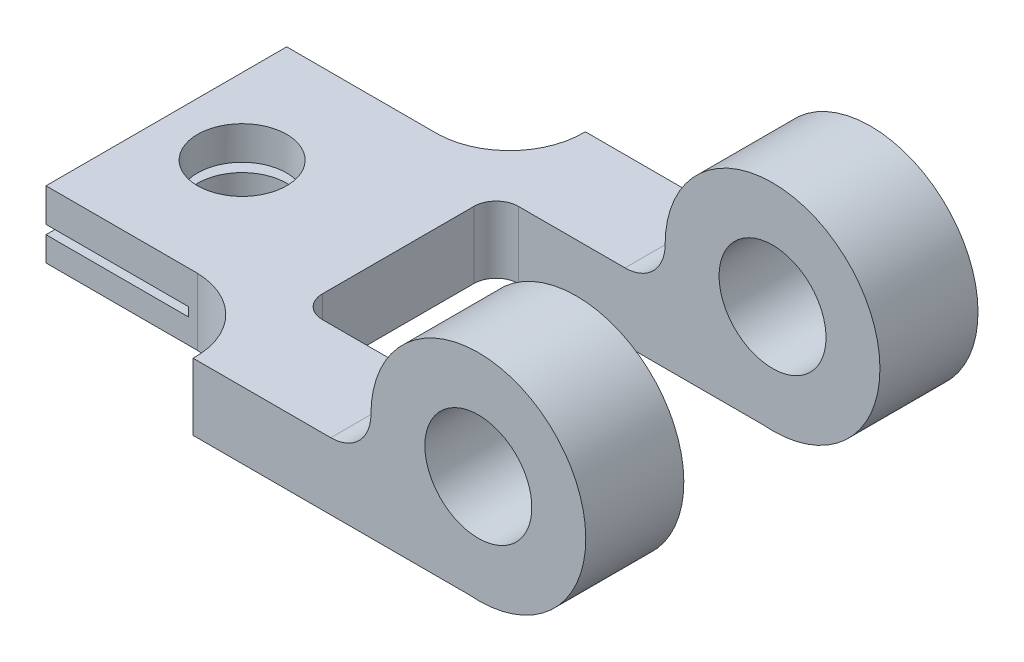
ISO-10303-21;
HEADER;
FILE_DESCRIPTION(('STEP AP214'),'2;1');
FILE_NAME('part.step','',(''),(''),'','','');
FILE_SCHEMA(('AUTOMOTIVE_DESIGN { 1 0 10303 214 1 1 1 1 }'));
ENDSEC;
DATA;
#1=APPLICATION_CONTEXT('core data for automotive mechanical design processes');
#2=APPLICATION_PROTOCOL_DEFINITION('international standard','automotive_design',2000,#1);
#3=PRODUCT_CONTEXT('',#1,'mechanical');
#4=PRODUCT('Part','Part','',(#3));
#5=PRODUCT_RELATED_PRODUCT_CATEGORY('part','',(#4));
#6=PRODUCT_DEFINITION_FORMATION('','',#4);
#7=PRODUCT_DEFINITION_CONTEXT('part definition',#1,'design');
#8=PRODUCT_DEFINITION('design','',#6,#7);
#9=PRODUCT_DEFINITION_SHAPE('','',#8);
#10=(LENGTH_UNIT() NAMED_UNIT(*) SI_UNIT(.MILLI.,.METRE.));
#11=(NAMED_UNIT(*) PLANE_ANGLE_UNIT() SI_UNIT($,.RADIAN.));
#12=(NAMED_UNIT(*) SI_UNIT($,.STERADIAN.) SOLID_ANGLE_UNIT());
#13=UNCERTAINTY_MEASURE_WITH_UNIT(LENGTH_MEASURE(1.E-05),#10,'distance_accuracy_value','');
#14=(GEOMETRIC_REPRESENTATION_CONTEXT(3) GLOBAL_UNCERTAINTY_ASSIGNED_CONTEXT((#13)) GLOBAL_UNIT_ASSIGNED_CONTEXT((#10,
#11,#12)) REPRESENTATION_CONTEXT('',''));
#15=CARTESIAN_POINT('',(0.,0.,0.));
#16=DIRECTION('',(0.,0.,1.));
#17=DIRECTION('',(1.,0.,0.));
#18=AXIS2_PLACEMENT_3D('',#15,#16,#17);
#19=CARTESIAN_POINT('',(-57.,15.,44.));
#20=DIRECTION('',(1.,0.,0.));
#21=DIRECTION('',(0.,0.,-1.));
#22=AXIS2_PLACEMENT_3D('',#19,#20,#21);
#23=PLANE('',#22);
#24=DIRECTION('',(0.,1.,0.));
#25=VECTOR('',#24,1.);
#26=CARTESIAN_POINT('',(-57.,-0.0999999999999959,27.));
#27=LINE('',#26,#25);
#28=CARTESIAN_POINT('',(-57.,0.,27.));
#29=VERTEX_POINT('',#28);
#30=CARTESIAN_POINT('',(-57.,5.5,27.));
#31=VERTEX_POINT('',#30);
#32=EDGE_CURVE('E240',#29,#31,#27,.T.);
#33=ORIENTED_EDGE('',*,*,#32,.T.);
#34=DIRECTION('',(0.,0.,-1.));
#35=VECTOR('',#34,1.);
#36=CARTESIAN_POINT('',(-57.,5.5,44.));
#37=LINE('',#36,#35);
#38=CARTESIAN_POINT('',(-57.,5.5,-27.));
#39=VERTEX_POINT('',#38);
#40=EDGE_CURVE('E189',#31,#39,#37,.T.);
#41=ORIENTED_EDGE('',*,*,#40,.T.);
#42=DIRECTION('',(0.,1.,0.));
#43=VECTOR('',#42,1.);
#44=CARTESIAN_POINT('',(-57.,-0.0999999999999959,-27.));
#45=LINE('',#44,#43);
#46=CARTESIAN_POINT('',(-57.,0.,-27.));
#47=VERTEX_POINT('',#46);
#48=EDGE_CURVE('E223',#47,#39,#45,.T.);
#49=ORIENTED_EDGE('',*,*,#48,.F.);
#50=DIRECTION('',(0.,0.,1.));
#51=VECTOR('',#50,1.);
#52=CARTESIAN_POINT('',(-57.,0.,44.));
#53=LINE('',#52,#51);
#54=EDGE_CURVE('E299',#47,#29,#53,.T.);
#55=ORIENTED_EDGE('',*,*,#54,.T.);
#56=EDGE_LOOP('',(#33,#41,#49,#55));
#57=FACE_BOUND('',#56,.T.);
#58=ADVANCED_FACE('F44',(#57),#23,.F.);
#59=CARTESIAN_POINT('',(-40.,-0.0999999999999959,0.));
#60=DIRECTION('',(0.,1.,0.));
#61=DIRECTION('',(0.,0.,1.));
#62=AXIS2_PLACEMENT_3D('',#59,#60,#61);
#63=CYLINDRICAL_SURFACE('',#62,10.);
#64=CARTESIAN_POINT('',(-40.,5.5,0.));
#65=DIRECTION('',(0.,-1.,0.));
#66=DIRECTION('',(1.,0.,0.));
#67=AXIS2_PLACEMENT_3D('',#64,#65,#66);
#68=CIRCLE('',#67,10.);
#69=CARTESIAN_POINT('',(-30.,5.5,0.));
#70=VERTEX_POINT('',#69);
#71=EDGE_CURVE('E202',#70,#70,#68,.F.);
#72=ORIENTED_EDGE('',*,*,#71,.T.);
#73=EDGE_LOOP('',(#72));
#74=FACE_BOUND('',#73,.T.);
#75=CARTESIAN_POINT('',(-40.,0.,0.));
#76=DIRECTION('',(0.,-1.,0.));
#77=DIRECTION('',(0.,0.,-1.));
#78=AXIS2_PLACEMENT_3D('',#75,#76,#77);
#79=CIRCLE('',#78,10.);
#80=CARTESIAN_POINT('',(-40.,0.,-10.));
#81=VERTEX_POINT('',#80);
#82=EDGE_CURVE('E270',#81,#81,#79,.T.);
#83=ORIENTED_EDGE('',*,*,#82,.T.);
#84=EDGE_LOOP('',(#83));
#85=FACE_BOUND('',#84,.T.);
#86=ADVANCED_FACE('F443',(#74,#85),#63,.F.);
#87=CARTESIAN_POINT('',(57.,24.,44.));
#88=DIRECTION('',(0.,0.,-1.));
#89=DIRECTION('',(-1.,0.,0.));
#90=AXIS2_PLACEMENT_3D('',#87,#88,#89);
#91=CYLINDRICAL_SURFACE('',#90,12.);
#92=CARTESIAN_POINT('',(57.,24.,44.));
#93=DIRECTION('',(0.,0.,-1.));
#94=DIRECTION('',(-1.,0.,0.));
#95=AXIS2_PLACEMENT_3D('',#92,#93,#94);
#96=CIRCLE('',#95,12.);
#97=CARTESIAN_POINT('',(45.,24.,44.));
#98=VERTEX_POINT('',#97);
#99=EDGE_CURVE('E268',#98,#98,#96,.T.);
#100=ORIENTED_EDGE('',*,*,#99,.F.);
#101=EDGE_LOOP('',(#100));
#102=FACE_BOUND('',#101,.T.);
#103=CARTESIAN_POINT('',(57.,24.,22.));
#104=DIRECTION('',(0.,0.,1.));
#105=DIRECTION('',(1.,0.,0.));
#106=AXIS2_PLACEMENT_3D('',#103,#104,#105);
#107=CIRCLE('',#106,12.);
#108=CARTESIAN_POINT('',(69.,24.,22.));
#109=VERTEX_POINT('',#108);
#110=EDGE_CURVE('E271',#109,#109,#107,.T.);
#111=ORIENTED_EDGE('',*,*,#110,.F.);
#112=EDGE_LOOP('',(#111));
#113=FACE_BOUND('',#112,.T.);
#114=ADVANCED_FACE('F445',(#102,#113),#91,.F.);
#115=CARTESIAN_POINT('',(-57.,15.,-44.));
#116=DIRECTION('',(0.,0.,1.));
#117=DIRECTION('',(1.,0.,0.));
#118=AXIS2_PLACEMENT_3D('',#115,#116,#117);
#119=PLANE('',#118);
#120=CARTESIAN_POINT('',(57.,24.,-44.));
#121=DIRECTION('',(0.,0.,-1.));
#122=DIRECTION('',(-1.,0.,0.));
#123=AXIS2_PLACEMENT_3D('',#120,#121,#122);
#124=CIRCLE('',#123,12.);
#125=CARTESIAN_POINT('',(45.,24.,-44.));
#126=VERTEX_POINT('',#125);
#127=EDGE_CURVE('E275',#126,#126,#124,.T.);
#128=ORIENTED_EDGE('',*,*,#127,.F.);
#129=EDGE_LOOP('',(#128));
#130=FACE_BOUND('',#129,.T.);
#131=DIRECTION('',(-1.,0.,0.));
#132=VECTOR('',#131,1.);
#133=CARTESIAN_POINT('',(-57.,0.,-44.));
#134=LINE('',#133,#132);
#135=CARTESIAN_POINT('',(54.8068287800539,0.,-44.));
#136=VERTEX_POINT('',#135);
#137=CARTESIAN_POINT('',(-6.99999999999999,0.,-44.));
#138=VERTEX_POINT('',#137);
#139=EDGE_CURVE('E284',#136,#138,#134,.T.);
#140=ORIENTED_EDGE('',*,*,#139,.T.);
#141=DIRECTION('',(0.,1.,0.));
#142=VECTOR('',#141,1.);
#143=CARTESIAN_POINT('',(-6.99999999999999,-0.0999999999999959,-44.));
#144=LINE('',#143,#142);
#145=CARTESIAN_POINT('',(-6.99999999999999,15.,-44.));
#146=VERTEX_POINT('',#145);
#147=EDGE_CURVE('E218',#138,#146,#144,.T.);
#148=ORIENTED_EDGE('',*,*,#147,.T.);
#149=DIRECTION('',(-1.,0.,0.));
#150=VECTOR('',#149,1.);
#151=CARTESIAN_POINT('',(-57.,15.,-44.));
#152=LINE('',#151,#150);
#153=CARTESIAN_POINT('',(23.9,15.,-44.));
#154=VERTEX_POINT('',#153);
#155=EDGE_CURVE('E287',#154,#146,#152,.T.);
#156=ORIENTED_EDGE('',*,*,#155,.F.);
#157=CARTESIAN_POINT('',(23.9,24.,-44.));
#158=DIRECTION('',(0.,0.,1.));
#159=DIRECTION('',(1.,0.,0.));
#160=AXIS2_PLACEMENT_3D('',#157,#158,#159);
#161=CIRCLE('',#160,9.);
#162=CARTESIAN_POINT('',(32.9,24.,-44.));
#163=VERTEX_POINT('',#162);
#164=EDGE_CURVE('E321',#154,#163,#161,.T.);
#165=ORIENTED_EDGE('',*,*,#164,.T.);
#166=CARTESIAN_POINT('',(57.,24.,-44.));
#167=DIRECTION('',(0.,0.,-1.));
#168=DIRECTION('',(-1.,0.,0.));
#169=AXIS2_PLACEMENT_3D('',#166,#167,#168);
#170=CIRCLE('',#169,24.1);
#171=EDGE_CURVE('E280',#163,#136,#170,.T.);
#172=ORIENTED_EDGE('',*,*,#171,.T.);
#173=EDGE_LOOP('',(#140,#148,#156,#165,#172));
#174=FACE_BOUND('',#173,.T.);
#175=ADVANCED_FACE('F387',(#130,#174),#119,.F.);
#176=CARTESIAN_POINT('',(-57.,7.5,-27.));
#177=VERTEX_POINT('',#176);
#178=CARTESIAN_POINT('',(-57.,15.,-27.));
#179=VERTEX_POINT('',#178);
#180=EDGE_CURVE('E217',#177,#179,#45,.T.);
#181=ORIENTED_EDGE('',*,*,#180,.F.);
#182=DIRECTION('',(0.,0.,-1.));
#183=VECTOR('',#182,1.);
#184=CARTESIAN_POINT('',(-57.,7.5,44.));
#185=LINE('',#184,#183);
#186=CARTESIAN_POINT('',(-57.,7.5,27.));
#187=VERTEX_POINT('',#186);
#188=EDGE_CURVE('E184',#187,#177,#185,.T.);
#189=ORIENTED_EDGE('',*,*,#188,.F.);
#190=CARTESIAN_POINT('',(-57.,15.,27.));
#191=VERTEX_POINT('',#190);
#192=EDGE_CURVE('E234',#187,#191,#27,.T.);
#193=ORIENTED_EDGE('',*,*,#192,.T.);
#194=DIRECTION('',(0.,0.,1.));
#195=VECTOR('',#194,1.);
#196=CARTESIAN_POINT('',(-57.,15.,44.));
#197=LINE('',#196,#195);
#198=EDGE_CURVE('E290',#179,#191,#197,.T.);
#199=ORIENTED_EDGE('',*,*,#198,.F.);
#200=EDGE_LOOP('',(#181,#189,#193,#199));
#201=FACE_BOUND('',#200,.T.);
#202=ADVANCED_FACE('F354',(#201),#23,.F.);
#203=CARTESIAN_POINT('',(-57.,15.,44.));
#204=DIRECTION('',(0.,0.,-1.));
#205=DIRECTION('',(-1.,0.,0.));
#206=AXIS2_PLACEMENT_3D('',#203,#204,#205);
#207=PLANE('',#206);
#208=ORIENTED_EDGE('',*,*,#99,.T.);
#209=EDGE_LOOP('',(#208));
#210=FACE_BOUND('',#209,.T.);
#211=DIRECTION('',(1.,0.,0.));
#212=VECTOR('',#211,1.);
#213=CARTESIAN_POINT('',(-57.,15.,44.));
#214=LINE('',#213,#212);
#215=CARTESIAN_POINT('',(-6.99999999999999,15.,44.));
#216=VERTEX_POINT('',#215);
#217=CARTESIAN_POINT('',(23.9,15.,44.));
#218=VERTEX_POINT('',#217);
#219=EDGE_CURVE('E294',#216,#218,#214,.T.);
#220=ORIENTED_EDGE('',*,*,#219,.F.);
#221=DIRECTION('',(0.,1.,0.));
#222=VECTOR('',#221,1.);
#223=CARTESIAN_POINT('',(-6.99999999999999,-0.0999999999999959,44.));
#224=LINE('',#223,#222);
#225=CARTESIAN_POINT('',(-6.99999999999999,0.,44.));
#226=VERTEX_POINT('',#225);
#227=EDGE_CURVE('E235',#226,#216,#224,.T.);
#228=ORIENTED_EDGE('',*,*,#227,.F.);
#229=DIRECTION('',(1.,0.,0.));
#230=VECTOR('',#229,1.);
#231=CARTESIAN_POINT('',(-57.,0.,44.));
#232=LINE('',#231,#230);
#233=CARTESIAN_POINT('',(54.8068287800539,0.,44.));
#234=VERTEX_POINT('',#233);
#235=EDGE_CURVE('E292',#226,#234,#232,.T.);
#236=ORIENTED_EDGE('',*,*,#235,.T.);
#237=CARTESIAN_POINT('',(57.,24.,44.));
#238=DIRECTION('',(0.,0.,1.));
#239=DIRECTION('',(1.,0.,0.));
#240=AXIS2_PLACEMENT_3D('',#237,#238,#239);
#241=CIRCLE('',#240,24.1);
#242=CARTESIAN_POINT('',(32.9,24.,44.));
#243=VERTEX_POINT('',#242);
#244=EDGE_CURVE('E278',#234,#243,#241,.T.);
#245=ORIENTED_EDGE('',*,*,#244,.T.);
#246=CARTESIAN_POINT('',(23.9,24.,44.));
#247=DIRECTION('',(0.,0.,-1.));
#248=DIRECTION('',(-1.,0.,0.));
#249=AXIS2_PLACEMENT_3D('',#246,#247,#248);
#250=CIRCLE('',#249,9.);
#251=EDGE_CURVE('E328',#243,#218,#250,.T.);
#252=ORIENTED_EDGE('',*,*,#251,.T.);
#253=EDGE_LOOP('',(#220,#228,#236,#245,#252));
#254=FACE_BOUND('',#253,.T.);
#255=ADVANCED_FACE('F430',(#210,#254),#207,.F.);
#256=CARTESIAN_POINT('',(0.,15.,0.));
#257=DIRECTION('',(0.,-1.,0.));
#258=DIRECTION('',(0.,0.,-1.));
#259=AXIS2_PLACEMENT_3D('',#256,#257,#258);
#260=PLANE('',#259);
#261=CARTESIAN_POINT('',(-40.,15.,0.));
#262=DIRECTION('',(0.,1.,0.));
#263=DIRECTION('',(0.,0.,1.));
#264=AXIS2_PLACEMENT_3D('',#261,#262,#263);
#265=CIRCLE('',#264,10.);
#266=CARTESIAN_POINT('',(-40.,15.,10.));
#267=VERTEX_POINT('',#266);
#268=EDGE_CURVE('E225',#267,#267,#265,.T.);
#269=ORIENTED_EDGE('',*,*,#268,.F.);
#270=EDGE_LOOP('',(#269));
#271=FACE_BOUND('',#270,.T.);
#272=DIRECTION('',(0.,0.,1.));
#273=VECTOR('',#272,1.);
#274=CARTESIAN_POINT('',(23.9,15.,0.));
#275=LINE('',#274,#273);
#276=CARTESIAN_POINT('',(23.9,15.,22.));
#277=VERTEX_POINT('',#276);
#278=EDGE_CURVE('E313',#218,#277,#275,.F.);
#279=ORIENTED_EDGE('',*,*,#278,.T.);
#280=DIRECTION('',(1.,0.,0.));
#281=VECTOR('',#280,1.);
#282=CARTESIAN_POINT('',(0.,15.,22.));
#283=LINE('',#282,#281);
#284=CARTESIAN_POINT('',(0.,15.,22.));
#285=VERTEX_POINT('',#284);
#286=EDGE_CURVE('E253',#285,#277,#283,.T.);
#287=ORIENTED_EDGE('',*,*,#286,.F.);
#288=CARTESIAN_POINT('',(0.,15.,17.));
#289=DIRECTION('',(0.,1.,0.));
#290=DIRECTION('',(0.,0.,1.));
#291=AXIS2_PLACEMENT_3D('',#288,#289,#290);
#292=CIRCLE('',#291,5.);
#293=CARTESIAN_POINT('',(-4.99999999999999,15.,17.));
#294=VERTEX_POINT('',#293);
#295=EDGE_CURVE('E249',#294,#285,#292,.T.);
#296=ORIENTED_EDGE('',*,*,#295,.F.);
#297=DIRECTION('',(0.,0.,1.));
#298=VECTOR('',#297,1.);
#299=CARTESIAN_POINT('',(-4.99999999999999,15.,-17.));
#300=LINE('',#299,#298);
#301=CARTESIAN_POINT('',(-4.99999999999999,15.,-17.));
#302=VERTEX_POINT('',#301);
#303=EDGE_CURVE('E241',#302,#294,#300,.T.);
#304=ORIENTED_EDGE('',*,*,#303,.F.);
#305=CARTESIAN_POINT('',(0.,15.,-17.));
#306=DIRECTION('',(0.,1.,0.));
#307=DIRECTION('',(0.,0.,1.));
#308=AXIS2_PLACEMENT_3D('',#305,#306,#307);
#309=CIRCLE('',#308,5.);
#310=CARTESIAN_POINT('',(0.,15.,-22.));
#311=VERTEX_POINT('',#310);
#312=EDGE_CURVE('E245',#311,#302,#309,.T.);
#313=ORIENTED_EDGE('',*,*,#312,.F.);
#314=DIRECTION('',(-1.,0.,0.));
#315=VECTOR('',#314,1.);
#316=CARTESIAN_POINT('',(57.,15.,-22.));
#317=LINE('',#316,#315);
#318=CARTESIAN_POINT('',(23.9,15.,-22.));
#319=VERTEX_POINT('',#318);
#320=EDGE_CURVE('E215',#319,#311,#317,.T.);
#321=ORIENTED_EDGE('',*,*,#320,.F.);
#322=DIRECTION('',(0.,0.,-1.));
#323=VECTOR('',#322,1.);
#324=CARTESIAN_POINT('',(23.9,15.,0.));
#325=LINE('',#324,#323);
#326=EDGE_CURVE('E314',#319,#154,#325,.T.);
#327=ORIENTED_EDGE('',*,*,#326,.T.);
#328=ORIENTED_EDGE('',*,*,#155,.T.);
#329=CARTESIAN_POINT('',(-23.5,15.,-43.5));
#330=DIRECTION('',(0.,1.,0.));
#331=DIRECTION('',(0.,0.,1.));
#332=AXIS2_PLACEMENT_3D('',#329,#330,#331);
#333=CIRCLE('',#332,16.5075740192192);
#334=CARTESIAN_POINT('',(-23.,15.,-27.));
#335=VERTEX_POINT('',#334);
#336=EDGE_CURVE('E216',#335,#146,#333,.T.);
#337=ORIENTED_EDGE('',*,*,#336,.F.);
#338=DIRECTION('',(1.,0.,0.));
#339=VECTOR('',#338,1.);
#340=CARTESIAN_POINT('',(-57.,15.,-27.));
#341=LINE('',#340,#339);
#342=EDGE_CURVE('E213',#179,#335,#341,.T.);
#343=ORIENTED_EDGE('',*,*,#342,.F.);
#344=ORIENTED_EDGE('',*,*,#198,.T.);
#345=DIRECTION('',(-1.,0.,0.));
#346=VECTOR('',#345,1.);
#347=CARTESIAN_POINT('',(-57.,15.,27.));
#348=LINE('',#347,#346);
#349=CARTESIAN_POINT('',(-23.,15.,27.));
#350=VERTEX_POINT('',#349);
#351=EDGE_CURVE('E230',#350,#191,#348,.T.);
#352=ORIENTED_EDGE('',*,*,#351,.F.);
#353=CARTESIAN_POINT('',(-23.5,15.,43.5));
#354=DIRECTION('',(0.,1.,0.));
#355=DIRECTION('',(0.,0.,-1.));
#356=AXIS2_PLACEMENT_3D('',#353,#354,#355);
#357=CIRCLE('',#356,16.5075740192192);
#358=EDGE_CURVE('E226',#216,#350,#357,.T.);
#359=ORIENTED_EDGE('',*,*,#358,.F.);
#360=ORIENTED_EDGE('',*,*,#219,.T.);
#361=EDGE_LOOP('',(#279,#287,#296,#304,#313,#321,#327,#328,#337,#343,#344,#352,#359,#360));
#362=FACE_BOUND('',#361,.T.);
#363=ADVANCED_FACE('F377',(#271,#362),#260,.F.);
#364=CARTESIAN_POINT('',(0.,0.,0.));
#365=DIRECTION('',(0.,-1.,0.));
#366=DIRECTION('',(0.,0.,-1.));
#367=AXIS2_PLACEMENT_3D('',#364,#365,#366);
#368=PLANE('',#367);
#369=DIRECTION('',(-1.,0.,0.));
#370=VECTOR('',#369,1.);
#371=CARTESIAN_POINT('',(0.,0.,22.));
#372=LINE('',#371,#370);
#373=CARTESIAN_POINT('',(54.8068287800539,0.,22.));
#374=VERTEX_POINT('',#373);
#375=CARTESIAN_POINT('',(0.,0.,22.));
#376=VERTEX_POINT('',#375);
#377=EDGE_CURVE('E265',#374,#376,#372,.T.);
#378=ORIENTED_EDGE('',*,*,#377,.F.);
#379=DIRECTION('',(0.,0.,1.));
#380=VECTOR('',#379,1.);
#381=CARTESIAN_POINT('',(54.8068287800539,0.,22.));
#382=LINE('',#381,#380);
#383=EDGE_CURVE('E297',#234,#374,#382,.F.);
#384=ORIENTED_EDGE('',*,*,#383,.F.);
#385=ORIENTED_EDGE('',*,*,#235,.F.);
#386=CARTESIAN_POINT('',(-23.5,0.,43.5));
#387=DIRECTION('',(0.,-1.,0.));
#388=DIRECTION('',(0.,0.,-1.));
#389=AXIS2_PLACEMENT_3D('',#386,#387,#388);
#390=CIRCLE('',#389,16.5075740192192);
#391=CARTESIAN_POINT('',(-23.,0.,27.));
#392=VERTEX_POINT('',#391);
#393=EDGE_CURVE('E339',#392,#226,#390,.T.);
#394=ORIENTED_EDGE('',*,*,#393,.F.);
#395=DIRECTION('',(1.,0.,0.));
#396=VECTOR('',#395,1.);
#397=CARTESIAN_POINT('',(0.,0.,27.));
#398=LINE('',#397,#396);
#399=EDGE_CURVE('E341',#29,#392,#398,.T.);
#400=ORIENTED_EDGE('',*,*,#399,.F.);
#401=ORIENTED_EDGE('',*,*,#54,.F.);
#402=DIRECTION('',(-1.,0.,0.));
#403=VECTOR('',#402,1.);
#404=CARTESIAN_POINT('',(0.,0.,-27.));
#405=LINE('',#404,#403);
#406=CARTESIAN_POINT('',(-23.,0.,-27.));
#407=VERTEX_POINT('',#406);
#408=EDGE_CURVE('E335',#407,#47,#405,.T.);
#409=ORIENTED_EDGE('',*,*,#408,.F.);
#410=CARTESIAN_POINT('',(-23.5,0.,-43.5));
#411=DIRECTION('',(0.,-1.,0.));
#412=DIRECTION('',(0.,0.,-1.));
#413=AXIS2_PLACEMENT_3D('',#410,#411,#412);
#414=CIRCLE('',#413,16.5075740192192);
#415=EDGE_CURVE('E337',#138,#407,#414,.T.);
#416=ORIENTED_EDGE('',*,*,#415,.F.);
#417=ORIENTED_EDGE('',*,*,#139,.F.);
#418=DIRECTION('',(0.,0.,-1.));
#419=VECTOR('',#418,1.);
#420=CARTESIAN_POINT('',(54.8068287800539,0.,-22.));
#421=LINE('',#420,#419);
#422=CARTESIAN_POINT('',(54.8068287800539,0.,-22.));
#423=VERTEX_POINT('',#422);
#424=EDGE_CURVE('E305',#423,#136,#421,.T.);
#425=ORIENTED_EDGE('',*,*,#424,.F.);
#426=DIRECTION('',(1.,0.,0.));
#427=VECTOR('',#426,1.);
#428=CARTESIAN_POINT('',(0.,0.,-22.));
#429=LINE('',#428,#427);
#430=CARTESIAN_POINT('',(0.,0.,-22.));
#431=VERTEX_POINT('',#430);
#432=EDGE_CURVE('E262',#431,#423,#429,.T.);
#433=ORIENTED_EDGE('',*,*,#432,.F.);
#434=CARTESIAN_POINT('',(0.,0.,-17.));
#435=DIRECTION('',(0.,-1.,0.));
#436=DIRECTION('',(0.,0.,-1.));
#437=AXIS2_PLACEMENT_3D('',#434,#435,#436);
#438=CIRCLE('',#437,5.);
#439=CARTESIAN_POINT('',(-4.99999999999999,0.,-17.));
#440=VERTEX_POINT('',#439);
#441=EDGE_CURVE('E344',#440,#431,#438,.T.);
#442=ORIENTED_EDGE('',*,*,#441,.F.);
#443=DIRECTION('',(0.,0.,-1.));
#444=VECTOR('',#443,1.);
#445=CARTESIAN_POINT('',(-4.99999999999999,0.,0.));
#446=LINE('',#445,#444);
#447=CARTESIAN_POINT('',(-4.99999999999999,0.,17.));
#448=VERTEX_POINT('',#447);
#449=EDGE_CURVE('E345',#448,#440,#446,.T.);
#450=ORIENTED_EDGE('',*,*,#449,.F.);
#451=CARTESIAN_POINT('',(0.,0.,17.));
#452=DIRECTION('',(0.,-1.,0.));
#453=DIRECTION('',(0.,0.,-1.));
#454=AXIS2_PLACEMENT_3D('',#451,#452,#453);
#455=CIRCLE('',#454,5.);
#456=EDGE_CURVE('E350',#376,#448,#455,.T.);
#457=ORIENTED_EDGE('',*,*,#456,.F.);
#458=EDGE_LOOP('',(#378,#384,#385,#394,#400,#401,#409,#416,#417,#425,#433,#442,#450,#457));
#459=FACE_BOUND('',#458,.T.);
#460=ORIENTED_EDGE('',*,*,#82,.F.);
#461=EDGE_LOOP('',(#460));
#462=FACE_BOUND('',#461,.T.);
#463=ADVANCED_FACE('F370',(#459,#462),#368,.T.);
#464=CARTESIAN_POINT('',(57.,24.,22.));
#465=DIRECTION('',(0.,0.,1.));
#466=DIRECTION('',(1.,0.,0.));
#467=AXIS2_PLACEMENT_3D('',#464,#465,#466);
#468=CYLINDRICAL_SURFACE('',#467,24.1);
#469=CARTESIAN_POINT('',(57.,24.,22.));
#470=DIRECTION('',(0.,0.,1.));
#471=DIRECTION('',(1.,0.,0.));
#472=AXIS2_PLACEMENT_3D('',#469,#470,#471);
#473=CIRCLE('',#472,24.1);
#474=CARTESIAN_POINT('',(32.9,24.,22.));
#475=VERTEX_POINT('',#474);
#476=EDGE_CURVE('E285',#374,#475,#473,.T.);
#477=ORIENTED_EDGE('',*,*,#476,.T.);
#478=DIRECTION('',(0.,0.,1.));
#479=VECTOR('',#478,1.);
#480=CARTESIAN_POINT('',(32.9,24.,22.));
#481=LINE('',#480,#479);
#482=EDGE_CURVE('E317',#475,#243,#481,.T.);
#483=ORIENTED_EDGE('',*,*,#482,.T.);
#484=ORIENTED_EDGE('',*,*,#244,.F.);
#485=ORIENTED_EDGE('',*,*,#383,.T.);
#486=EDGE_LOOP('',(#477,#483,#484,#485));
#487=FACE_BOUND('',#486,.T.);
#488=ADVANCED_FACE('F421',(#487),#468,.T.);
#489=CARTESIAN_POINT('',(57.,24.,22.));
#490=DIRECTION('',(0.,0.,1.));
#491=DIRECTION('',(1.,0.,0.));
#492=AXIS2_PLACEMENT_3D('',#489,#490,#491);
#493=PLANE('',#492);
#494=ORIENTED_EDGE('',*,*,#476,.F.);
#495=ORIENTED_EDGE('',*,*,#377,.T.);
#496=DIRECTION('',(0.,1.,0.));
#497=VECTOR('',#496,1.);
#498=CARTESIAN_POINT('',(0.,-0.0999999999999959,22.));
#499=LINE('',#498,#497);
#500=EDGE_CURVE('E231',#376,#285,#499,.T.);
#501=ORIENTED_EDGE('',*,*,#500,.T.);
#502=ORIENTED_EDGE('',*,*,#286,.T.);
#503=CARTESIAN_POINT('',(23.9,24.,22.));
#504=DIRECTION('',(0.,0.,1.));
#505=DIRECTION('',(1.,0.,0.));
#506=AXIS2_PLACEMENT_3D('',#503,#504,#505);
#507=CIRCLE('',#506,9.);
#508=EDGE_CURVE('E326',#277,#475,#507,.T.);
#509=ORIENTED_EDGE('',*,*,#508,.T.);
#510=EDGE_LOOP('',(#494,#495,#501,#502,#509));
#511=FACE_BOUND('',#510,.T.);
#512=ORIENTED_EDGE('',*,*,#110,.T.);
#513=EDGE_LOOP('',(#512));
#514=FACE_BOUND('',#513,.T.);
#515=ADVANCED_FACE('F417',(#511,#514),#493,.F.);
#516=CARTESIAN_POINT('',(57.,24.,-22.));
#517=DIRECTION('',(0.,0.,-1.));
#518=DIRECTION('',(-1.,0.,0.));
#519=AXIS2_PLACEMENT_3D('',#516,#517,#518);
#520=CYLINDRICAL_SURFACE('',#519,24.1);
#521=ORIENTED_EDGE('',*,*,#171,.F.);
#522=DIRECTION('',(0.,0.,-1.));
#523=VECTOR('',#522,1.);
#524=CARTESIAN_POINT('',(32.9,24.,-22.));
#525=LINE('',#524,#523);
#526=CARTESIAN_POINT('',(32.9,24.,-22.));
#527=VERTEX_POINT('',#526);
#528=EDGE_CURVE('E320',#163,#527,#525,.F.);
#529=ORIENTED_EDGE('',*,*,#528,.T.);
#530=CARTESIAN_POINT('',(57.,24.,-22.));
#531=DIRECTION('',(0.,0.,-1.));
#532=DIRECTION('',(-1.,0.,0.));
#533=AXIS2_PLACEMENT_3D('',#530,#531,#532);
#534=CIRCLE('',#533,24.1);
#535=EDGE_CURVE('E279',#527,#423,#534,.T.);
#536=ORIENTED_EDGE('',*,*,#535,.T.);
#537=ORIENTED_EDGE('',*,*,#424,.T.);
#538=EDGE_LOOP('',(#521,#529,#536,#537));
#539=FACE_BOUND('',#538,.T.);
#540=ADVANCED_FACE('F395',(#539),#520,.T.);
#541=CARTESIAN_POINT('',(57.,24.,-22.));
#542=DIRECTION('',(0.,0.,-1.));
#543=DIRECTION('',(-1.,0.,0.));
#544=AXIS2_PLACEMENT_3D('',#541,#542,#543);
#545=PLANE('',#544);
#546=ORIENTED_EDGE('',*,*,#432,.T.);
#547=ORIENTED_EDGE('',*,*,#535,.F.);
#548=CARTESIAN_POINT('',(23.9,24.,-22.));
#549=DIRECTION('',(0.,0.,-1.));
#550=DIRECTION('',(-1.,0.,0.));
#551=AXIS2_PLACEMENT_3D('',#548,#549,#550);
#552=CIRCLE('',#551,9.);
#553=EDGE_CURVE('E323',#527,#319,#552,.T.);
#554=ORIENTED_EDGE('',*,*,#553,.T.);
#555=ORIENTED_EDGE('',*,*,#320,.T.);
#556=DIRECTION('',(0.,1.,0.));
#557=VECTOR('',#556,1.);
#558=CARTESIAN_POINT('',(0.,-0.0999999999999959,-22.));
#559=LINE('',#558,#557);
#560=EDGE_CURVE('E251',#431,#311,#559,.T.);
#561=ORIENTED_EDGE('',*,*,#560,.F.);
#562=EDGE_LOOP('',(#546,#547,#554,#555,#561));
#563=FACE_BOUND('',#562,.T.);
#564=CARTESIAN_POINT('',(57.,24.,-22.));
#565=DIRECTION('',(0.,0.,-1.));
#566=DIRECTION('',(-1.,0.,0.));
#567=AXIS2_PLACEMENT_3D('',#564,#565,#566);
#568=CIRCLE('',#567,12.);
#569=CARTESIAN_POINT('',(45.,24.,-22.));
#570=VERTEX_POINT('',#569);
#571=EDGE_CURVE('E306',#570,#570,#568,.T.);
#572=ORIENTED_EDGE('',*,*,#571,.T.);
#573=EDGE_LOOP('',(#572));
#574=FACE_BOUND('',#573,.T.);
#575=ADVANCED_FACE('F399',(#563,#574),#545,.F.);
#576=ORIENTED_EDGE('',*,*,#127,.T.);
#577=EDGE_LOOP('',(#576));
#578=FACE_BOUND('',#577,.T.);
#579=ORIENTED_EDGE('',*,*,#571,.F.);
#580=EDGE_LOOP('',(#579));
#581=FACE_BOUND('',#580,.T.);
#582=ADVANCED_FACE('F432',(#578,#581),#91,.F.);
#583=CARTESIAN_POINT('',(23.9,24.,-22.));
#584=DIRECTION('',(0.,0.,-1.));
#585=DIRECTION('',(-1.,0.,0.));
#586=AXIS2_PLACEMENT_3D('',#583,#584,#585);
#587=CYLINDRICAL_SURFACE('',#586,9.);
#588=ORIENTED_EDGE('',*,*,#553,.F.);
#589=ORIENTED_EDGE('',*,*,#528,.F.);
#590=ORIENTED_EDGE('',*,*,#164,.F.);
#591=ORIENTED_EDGE('',*,*,#326,.F.);
#592=EDGE_LOOP('',(#588,#589,#590,#591));
#593=FACE_BOUND('',#592,.T.);
#594=ADVANCED_FACE('F435',(#593),#587,.F.);
#595=CARTESIAN_POINT('',(23.9,24.,22.));
#596=DIRECTION('',(0.,0.,1.));
#597=DIRECTION('',(1.,0.,0.));
#598=AXIS2_PLACEMENT_3D('',#595,#596,#597);
#599=CYLINDRICAL_SURFACE('',#598,9.);
#600=ORIENTED_EDGE('',*,*,#251,.F.);
#601=ORIENTED_EDGE('',*,*,#482,.F.);
#602=ORIENTED_EDGE('',*,*,#508,.F.);
#603=ORIENTED_EDGE('',*,*,#278,.F.);
#604=EDGE_LOOP('',(#600,#601,#602,#603));
#605=FACE_BOUND('',#604,.T.);
#606=ADVANCED_FACE('F50',(#605),#599,.F.);
#607=CARTESIAN_POINT('',(0.,-0.0999999999999959,17.));
#608=DIRECTION('',(0.,1.,0.));
#609=DIRECTION('',(0.,0.,1.));
#610=AXIS2_PLACEMENT_3D('',#607,#608,#609);
#611=CYLINDRICAL_SURFACE('',#610,5.);
#612=ORIENTED_EDGE('',*,*,#456,.T.);
#613=DIRECTION('',(0.,1.,0.));
#614=VECTOR('',#613,1.);
#615=CARTESIAN_POINT('',(-4.99999999999999,-0.0999999999999959,17.));
#616=LINE('',#615,#614);
#617=EDGE_CURVE('E254',#448,#294,#616,.T.);
#618=ORIENTED_EDGE('',*,*,#617,.T.);
#619=ORIENTED_EDGE('',*,*,#295,.T.);
#620=ORIENTED_EDGE('',*,*,#500,.F.);
#621=EDGE_LOOP('',(#612,#618,#619,#620));
#622=FACE_BOUND('',#621,.T.);
#623=ADVANCED_FACE('F412',(#622),#611,.F.);
#624=CARTESIAN_POINT('',(-4.99999999999999,-0.0999999999999959,-17.));
#625=DIRECTION('',(-1.,0.,0.));
#626=DIRECTION('',(0.,0.,1.));
#627=AXIS2_PLACEMENT_3D('',#624,#625,#626);
#628=PLANE('',#627);
#629=ORIENTED_EDGE('',*,*,#449,.T.);
#630=DIRECTION('',(0.,1.,0.));
#631=VECTOR('',#630,1.);
#632=CARTESIAN_POINT('',(-4.99999999999999,-0.0999999999999959,-17.));
#633=LINE('',#632,#631);
#634=EDGE_CURVE('E260',#440,#302,#633,.T.);
#635=ORIENTED_EDGE('',*,*,#634,.T.);
#636=ORIENTED_EDGE('',*,*,#303,.T.);
#637=ORIENTED_EDGE('',*,*,#617,.F.);
#638=EDGE_LOOP('',(#629,#635,#636,#637));
#639=FACE_BOUND('',#638,.T.);
#640=ADVANCED_FACE('F409',(#639),#628,.F.);
#641=CARTESIAN_POINT('',(0.,-0.0999999999999959,-17.));
#642=DIRECTION('',(0.,1.,0.));
#643=DIRECTION('',(0.,0.,1.));
#644=AXIS2_PLACEMENT_3D('',#641,#642,#643);
#645=CYLINDRICAL_SURFACE('',#644,5.);
#646=ORIENTED_EDGE('',*,*,#441,.T.);
#647=ORIENTED_EDGE('',*,*,#560,.T.);
#648=ORIENTED_EDGE('',*,*,#312,.T.);
#649=ORIENTED_EDGE('',*,*,#634,.F.);
#650=EDGE_LOOP('',(#646,#647,#648,#649));
#651=FACE_BOUND('',#650,.T.);
#652=ADVANCED_FACE('F405',(#651),#645,.F.);
#653=CARTESIAN_POINT('',(-40.,7.5,0.));
#654=DIRECTION('',(0.,1.,0.));
#655=DIRECTION('',(-1.,0.,0.));
#656=AXIS2_PLACEMENT_3D('',#653,#654,#655);
#657=CIRCLE('',#656,10.);
#658=CARTESIAN_POINT('',(-50.,7.5,0.));
#659=VERTEX_POINT('',#658);
#660=EDGE_CURVE('E188',#659,#659,#657,.F.);
#661=ORIENTED_EDGE('',*,*,#660,.T.);
#662=EDGE_LOOP('',(#661));
#663=FACE_BOUND('',#662,.T.);
#664=ORIENTED_EDGE('',*,*,#268,.T.);
#665=EDGE_LOOP('',(#664));
#666=FACE_BOUND('',#665,.T.);
#667=ADVANCED_FACE('F453',(#663,#666),#63,.F.);
#668=CARTESIAN_POINT('',(-23.5,-0.0999999999999959,-43.5));
#669=DIRECTION('',(0.,1.,0.));
#670=DIRECTION('',(0.,0.,1.));
#671=AXIS2_PLACEMENT_3D('',#668,#669,#670);
#672=CYLINDRICAL_SURFACE('',#671,16.5075740192192);
#673=ORIENTED_EDGE('',*,*,#415,.T.);
#674=DIRECTION('',(0.,1.,0.));
#675=VECTOR('',#674,1.);
#676=CARTESIAN_POINT('',(-23.,-0.0999999999999959,-27.));
#677=LINE('',#676,#675);
#678=EDGE_CURVE('E224',#407,#335,#677,.T.);
#679=ORIENTED_EDGE('',*,*,#678,.T.);
#680=ORIENTED_EDGE('',*,*,#336,.T.);
#681=ORIENTED_EDGE('',*,*,#147,.F.);
#682=EDGE_LOOP('',(#673,#679,#680,#681));
#683=FACE_BOUND('',#682,.T.);
#684=ADVANCED_FACE('F383',(#683),#672,.F.);
#685=CARTESIAN_POINT('',(-57.,-0.0999999999999959,-27.));
#686=DIRECTION('',(0.,0.,1.));
#687=DIRECTION('',(1.,0.,0.));
#688=AXIS2_PLACEMENT_3D('',#685,#686,#687);
#689=PLANE('',#688);
#690=ORIENTED_EDGE('',*,*,#48,.T.);
#691=DIRECTION('',(1.,0.,0.));
#692=VECTOR('',#691,1.);
#693=CARTESIAN_POINT('',(-57.,5.5,-27.));
#694=LINE('',#693,#692);
#695=CARTESIAN_POINT('',(-25.,5.5,-27.));
#696=VERTEX_POINT('',#695);
#697=EDGE_CURVE('E201',#39,#696,#694,.T.);
#698=ORIENTED_EDGE('',*,*,#697,.T.);
#699=DIRECTION('',(0.,1.,0.));
#700=VECTOR('',#699,1.);
#701=CARTESIAN_POINT('',(-25.,-0.0999999999999959,-27.));
#702=LINE('',#701,#700);
#703=CARTESIAN_POINT('',(-25.,7.5,-27.));
#704=VERTEX_POINT('',#703);
#705=EDGE_CURVE('E193',#696,#704,#702,.T.);
#706=ORIENTED_EDGE('',*,*,#705,.T.);
#707=DIRECTION('',(-1.,0.,0.));
#708=VECTOR('',#707,1.);
#709=CARTESIAN_POINT('',(-57.,7.5,-27.));
#710=LINE('',#709,#708);
#711=EDGE_CURVE('E180',#704,#177,#710,.T.);
#712=ORIENTED_EDGE('',*,*,#711,.T.);
#713=ORIENTED_EDGE('',*,*,#180,.T.);
#714=ORIENTED_EDGE('',*,*,#342,.T.);
#715=ORIENTED_EDGE('',*,*,#678,.F.);
#716=ORIENTED_EDGE('',*,*,#408,.T.);
#717=EDGE_LOOP('',(#690,#698,#706,#712,#713,#714,#715,#716));
#718=FACE_BOUND('',#717,.T.);
#719=ADVANCED_FACE('F205',(#718),#689,.F.);
#720=CARTESIAN_POINT('',(-57.,-0.0999999999999959,27.));
#721=DIRECTION('',(0.,0.,-1.));
#722=DIRECTION('',(-1.,0.,0.));
#723=AXIS2_PLACEMENT_3D('',#720,#721,#722);
#724=PLANE('',#723);
#725=DIRECTION('',(0.,-1.,0.));
#726=VECTOR('',#725,1.);
#727=CARTESIAN_POINT('',(-25.,-0.0999999999999959,27.));
#728=LINE('',#727,#726);
#729=CARTESIAN_POINT('',(-25.,7.5,27.));
#730=VERTEX_POINT('',#729);
#731=CARTESIAN_POINT('',(-25.,5.5,27.));
#732=VERTEX_POINT('',#731);
#733=EDGE_CURVE('E52',#730,#732,#728,.T.);
#734=ORIENTED_EDGE('',*,*,#733,.T.);
#735=DIRECTION('',(-1.,0.,0.));
#736=VECTOR('',#735,1.);
#737=CARTESIAN_POINT('',(-57.,5.5,27.));
#738=LINE('',#737,#736);
#739=EDGE_CURVE('E11',#732,#31,#738,.T.);
#740=ORIENTED_EDGE('',*,*,#739,.T.);
#741=ORIENTED_EDGE('',*,*,#32,.F.);
#742=ORIENTED_EDGE('',*,*,#399,.T.);
#743=DIRECTION('',(0.,1.,0.));
#744=VECTOR('',#743,1.);
#745=CARTESIAN_POINT('',(-23.,-0.0999999999999959,27.));
#746=LINE('',#745,#744);
#747=EDGE_CURVE('E69',#392,#350,#746,.T.);
#748=ORIENTED_EDGE('',*,*,#747,.T.);
#749=ORIENTED_EDGE('',*,*,#351,.T.);
#750=ORIENTED_EDGE('',*,*,#192,.F.);
#751=DIRECTION('',(1.,0.,0.));
#752=VECTOR('',#751,1.);
#753=CARTESIAN_POINT('',(-57.,7.5,27.));
#754=LINE('',#753,#752);
#755=EDGE_CURVE('E349',#187,#730,#754,.T.);
#756=ORIENTED_EDGE('',*,*,#755,.T.);
#757=EDGE_LOOP('',(#734,#740,#741,#742,#748,#749,#750,#756));
#758=FACE_BOUND('',#757,.T.);
#759=ADVANCED_FACE('F352',(#758),#724,.F.);
#760=CARTESIAN_POINT('',(-23.5,-0.0999999999999959,43.5));
#761=DIRECTION('',(0.,1.,0.));
#762=DIRECTION('',(0.,0.,1.));
#763=AXIS2_PLACEMENT_3D('',#760,#761,#762);
#764=CYLINDRICAL_SURFACE('',#763,16.5075740192192);
#765=ORIENTED_EDGE('',*,*,#393,.T.);
#766=ORIENTED_EDGE('',*,*,#227,.T.);
#767=ORIENTED_EDGE('',*,*,#358,.T.);
#768=ORIENTED_EDGE('',*,*,#747,.F.);
#769=EDGE_LOOP('',(#765,#766,#767,#768));
#770=FACE_BOUND('',#769,.T.);
#771=ADVANCED_FACE('F374',(#770),#764,.F.);
#772=CARTESIAN_POINT('',(-57.,5.5,44.));
#773=DIRECTION('',(0.,-1.,0.));
#774=DIRECTION('',(1.,0.,0.));
#775=AXIS2_PLACEMENT_3D('',#772,#773,#774);
#776=PLANE('',#775);
#777=ORIENTED_EDGE('',*,*,#40,.F.);
#778=ORIENTED_EDGE('',*,*,#739,.F.);
#779=DIRECTION('',(0.,0.,-1.));
#780=VECTOR('',#779,1.);
#781=CARTESIAN_POINT('',(-25.,5.5,44.));
#782=LINE('',#781,#780);
#783=EDGE_CURVE('E196',#732,#696,#782,.T.);
#784=ORIENTED_EDGE('',*,*,#783,.T.);
#785=ORIENTED_EDGE('',*,*,#697,.F.);
#786=EDGE_LOOP('',(#777,#778,#784,#785));
#787=FACE_BOUND('',#786,.T.);
#788=ORIENTED_EDGE('',*,*,#71,.F.);
#789=EDGE_LOOP('',(#788));
#790=FACE_BOUND('',#789,.T.);
#791=ADVANCED_FACE('F597',(#787,#790),#776,.F.);
#792=CARTESIAN_POINT('',(-25.,5.5,44.));
#793=DIRECTION('',(1.,0.,0.));
#794=DIRECTION('',(0.,0.,-1.));
#795=AXIS2_PLACEMENT_3D('',#792,#793,#794);
#796=PLANE('',#795);
#797=ORIENTED_EDGE('',*,*,#783,.F.);
#798=ORIENTED_EDGE('',*,*,#733,.F.);
#799=DIRECTION('',(0.,0.,-1.));
#800=VECTOR('',#799,1.);
#801=CARTESIAN_POINT('',(-25.,7.5,44.));
#802=LINE('',#801,#800);
#803=EDGE_CURVE('E58',#730,#704,#802,.T.);
#804=ORIENTED_EDGE('',*,*,#803,.T.);
#805=ORIENTED_EDGE('',*,*,#705,.F.);
#806=EDGE_LOOP('',(#797,#798,#804,#805));
#807=FACE_BOUND('',#806,.T.);
#808=ADVANCED_FACE('F194',(#807),#796,.F.);
#809=CARTESIAN_POINT('',(-57.,7.5,44.));
#810=DIRECTION('',(0.,1.,0.));
#811=DIRECTION('',(-1.,0.,0.));
#812=AXIS2_PLACEMENT_3D('',#809,#810,#811);
#813=PLANE('',#812);
#814=ORIENTED_EDGE('',*,*,#803,.F.);
#815=ORIENTED_EDGE('',*,*,#755,.F.);
#816=ORIENTED_EDGE('',*,*,#188,.T.);
#817=ORIENTED_EDGE('',*,*,#711,.F.);
#818=EDGE_LOOP('',(#814,#815,#816,#817));
#819=FACE_BOUND('',#818,.T.);
#820=ORIENTED_EDGE('',*,*,#660,.F.);
#821=EDGE_LOOP('',(#820));
#822=FACE_BOUND('',#821,.T.);
#823=ADVANCED_FACE('F182',(#819,#822),#813,.F.);
#824=CLOSED_SHELL('',(#58,#86,#114,#175,#202,#255,#363,#463,#488,#515,#540,#575,#582,#594,#606,
#623,#640,#652,#667,#684,#719,#759,#771,#791,#808,#823));
#825=MANIFOLD_SOLID_BREP('B2',#824);
#826=ADVANCED_BREP_SHAPE_REPRESENTATION('',(#18,#825),#14);
#827=SHAPE_DEFINITION_REPRESENTATION(#9,#826);
ENDSEC;
END-ISO-10303-21;
